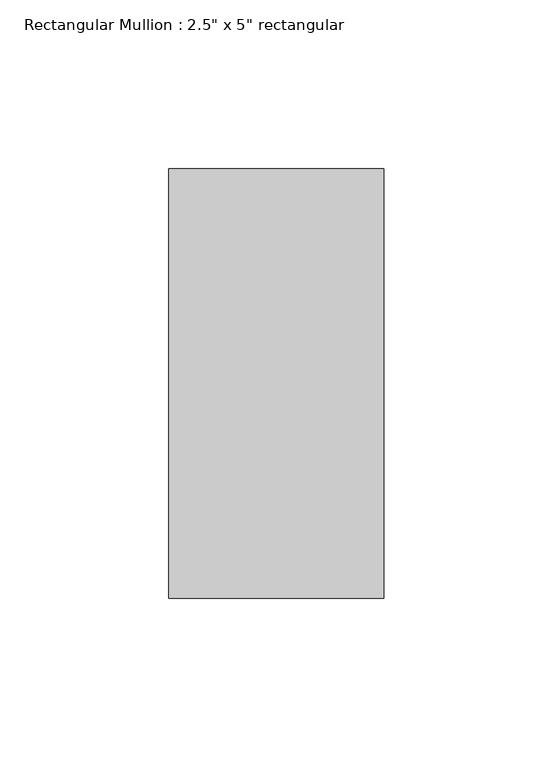
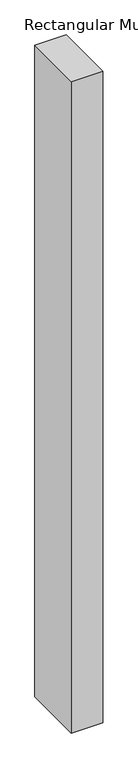
"""IFC4 building model written with IfcOpenShell, lengths in millimetres: member geometry."""

from ifc_helpers import new_model, si_unit, frame, origin, place, context, project, spatial, polyline, outline, extrude, source, transform, mapped, element, save


def member_11090e01(model_context):
    return source(origin(), model_context, "Body", "SweptSolid", [
        extrude(outline(polyline([(0.0, 63.5), (0.0, -63.5), (-63.5, -63.5), (-63.5, 63.5), (0.0, 63.5)])), frame((0.0, 0.0, -1387.9224956), z_axis=(0.0, 0.0, 1.0), x_axis=(1.0, 0.0, 0.0)), (0.0, 0.0, 1.0), 1387.9224956),
    ])


if __name__ == "__main__":
    model = new_model("IFC4")
    model_context = context("Model", 3, world=origin())
    ifc_project = project(units=[si_unit("LENGTHUNIT", "METRE", prefix="MILLI")], contexts=[model_context])
    site = spatial("IfcSite", under=ifc_project)
    building = spatial("IfcBuilding", under=site)
    placement = place(None, origin())
    member_shape = member_11090e01(model_context)
    element("IfcMember", 1, ObjectType="Rectangular Mullion : 2.5\" x 5\" rectangular", at=placement, inside=building, context=model_context, shape_type="MappedRepresentation", body=[
        mapped(member_shape, transform((0.0, 0.0, 0.0), x_axis=(1.0, 0.0, 0.0), y_axis=(0.0, 1.0, 0.0), z_axis=(0.0, 0.0, 1.0))),
    ])
    save(model, "model.ifc")

# Revit data of these elements
# Type "Rectangular Mullion : 2.5\" x 5\" rectangular"
#   built-in parameter 1007304 = 0.416667 (stored number, unit not read)
#   built-in parameter 1007301 = 0.104167 (stored number, unit not read)
#   built-in parameter 1007300 = 0.104167 (stored number, unit not read)
# Element 1 (IfcMember, "Rectangular Mullion : 2.5\" x 5\" rectangular")
#   Materials on its faces: "BLACK COLOUR"
# Materials
#   "BLACK COLOUR": class "Generic", colour RGB 120 120 120, transparency 0, Cost = 0
